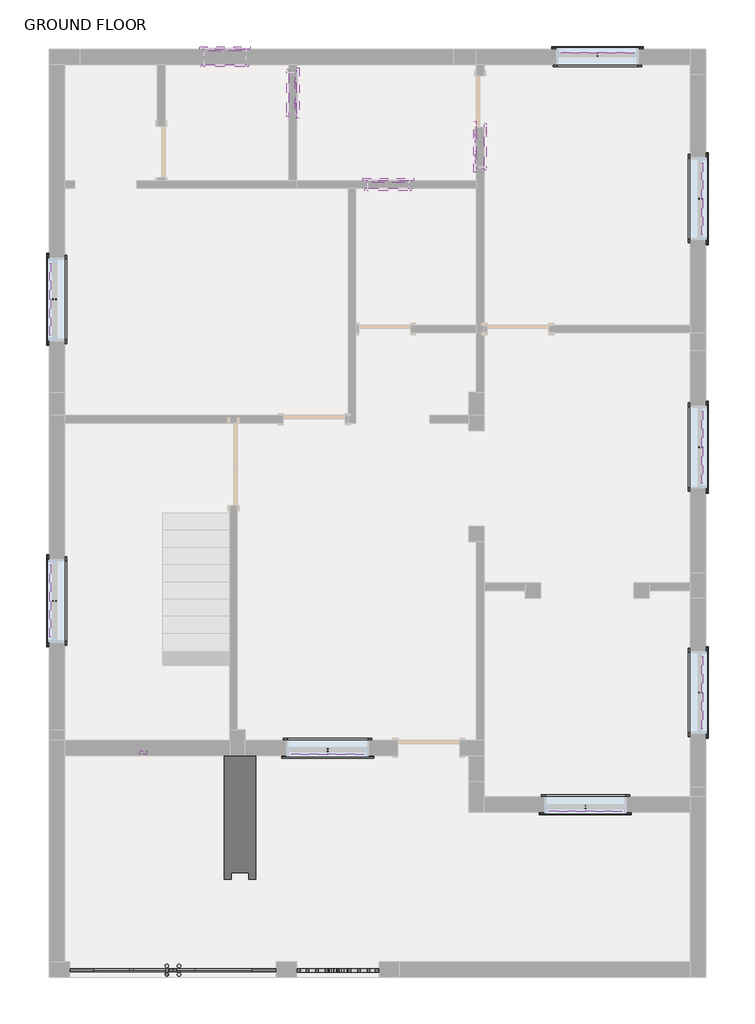
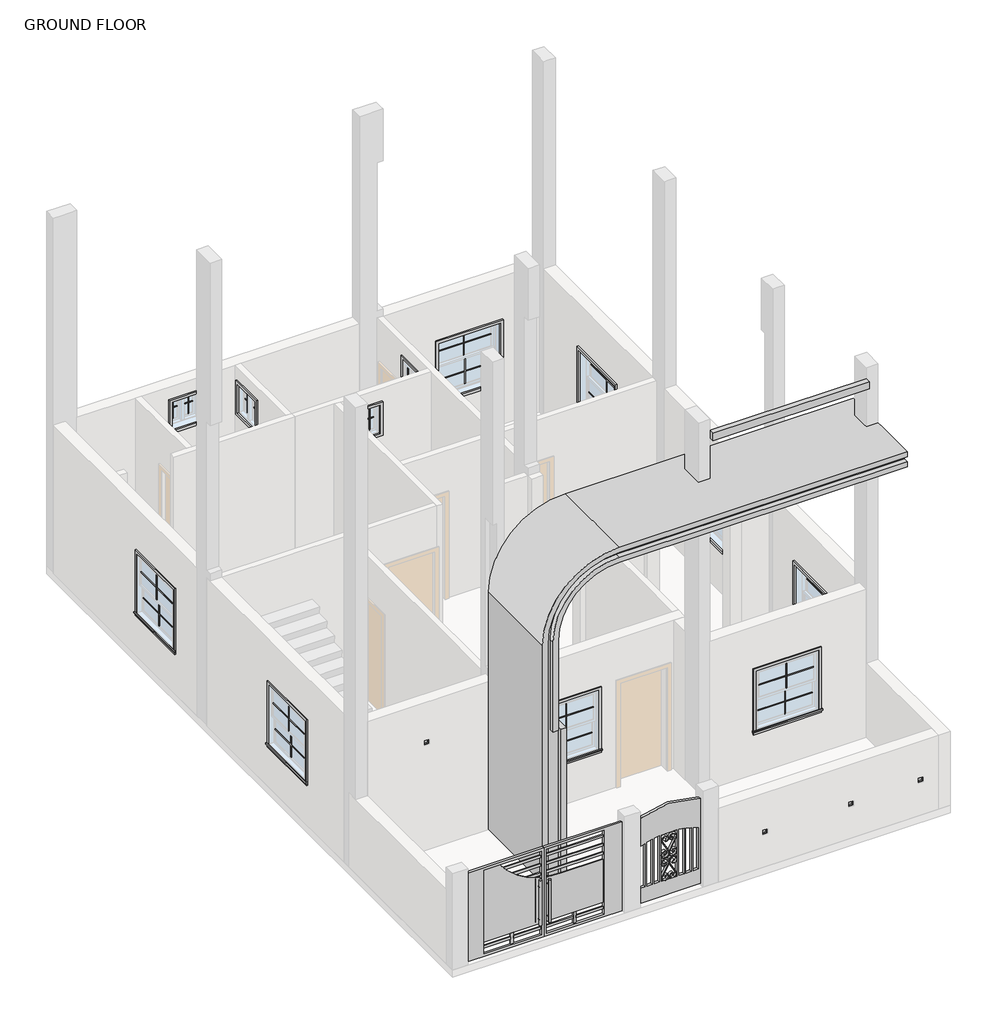
# One storey, part 3 of 3: 51 proxies, 4 light fixtures.
"""IFC4 building model written with IfcOpenShell, lengths in millimetres."""

from ifc_helpers import new_model, si_unit, frame, origin, place, context, project, spatial, polyline, circle_curve, outline, extrude, transform, mapped, element, save
from ifc_brep_helpers import plane_surface, cylinder_surface, revolved_surface, advanced_brep
from components import generic_models_d903a639, muntin_pattern_2x2_muntin_pattern_2x2_1e1a1b39, muntin_pattern_2x2_muntin_pattern_2x2_0961b91c, muntin_pattern_2x2_muntin_pattern_2x2_cae9449b, spanish_gate_w_wrought_iron_detail_3643_spanish_gate_w_2ba93c97, trim_window_exterior_flat_with_sill_7cfdd449, trim_window_exterior_flat_with_sill_858dc10d, trim_window_interior_flat_picture_frame_f1e0b15b, trim_window_interior_flat_picture_frame_3927330c, light_fixture_da35b629

model = new_model("IFC4")

# Units and contexts
model_context = context("Model", 3, world=origin())
ifc_project = project(units=[si_unit("LENGTHUNIT", "METRE", prefix="MILLI")], contexts=[model_context])

# Site, building, storey
site = spatial("IfcSite", under=ifc_project)
building = spatial("IfcBuilding", under=site)
storey = spatial("IfcBuildingStorey", under=building, Name="GROUND FLOOR", Elevation=0.0)

# Proxies
placement = place(None, origin())
generic_models_shape = generic_models_d903a639(model_context)
element("IfcBuildingElementProxy", 1, Name="Generic Models", at=placement, inside=storey, context=model_context, shape_type="MappedRepresentation", body=[
    mapped(generic_models_shape, transform((-11061.7029075, -4701.2829343, 0.0), x_axis=(1.0, 0.0, 0.0), y_axis=(0.0, 1.0, 0.0), z_axis=(0.0, 0.0, 1.0))),
])
element("IfcBuildingElementProxy", 2, Name="Generic Models 1 : Generic Models 1", ObjectType="Generic Models 1 : Generic Models 1", at=placement, inside=storey, context=model_context, shape_type="SolidModel", body=[
    extrude(outline(polyline([(-3417.2209734, -2491.4829343), (-6465.2209734, -2491.4829343), (-6465.2209734, -2389.8829343), (-3417.2209734, -2389.8829343), (-3417.2209734, -2491.4829343)])), frame((0.0, 0.0, 7239.8477718), z_axis=(0.0, 0.0, 1.0), x_axis=(1.0, 0.0, 0.0)), (0.0, 0.0, 1.0), 152.4),
    advanced_brep(
    [(-9837.0709734, -3380.4829343, 0.0), (-9837.0709734, -3380.4829343, 3048.0), (-9938.6709734, -3380.4829343, 3048.0), (-9938.6709734, -3380.4829343, 0.0), (-9837.0709734, -1551.6829343, 0.0), (-10300.6209734, -1551.6829343, 0.0), (-10300.6209734, -1551.6829343, 4902.2), (-8802.0209734, -1551.6829343, 6400.8), (-3188.6209734, -1551.6829343, 6400.8), (-3188.6209734, -1551.6829343, 6096.0), (-8802.0209734, -1551.6829343, 6096.0), (-9995.8209734, -1551.6829343, 4902.2), (-9995.8209734, -1551.6829343, 3048.0), (-9837.0709734, -1551.6829343, 3048.0), (-8802.0209734, -3380.4829343, 6096.0), (-9995.8209734, -3380.4829343, 4902.2), (-3188.6209734, -3380.4829343, 6096.0), (-3188.6209734, -3380.4829343, 6400.8), (-3188.6209734, -3380.4829343, 6299.2), (-3188.6209734, -3278.8829343, 6299.2), (-3188.6209734, -3278.8829343, 6197.6), (-3188.6209734, -3380.4829343, 6197.6), (-8802.0209734, -3380.4829343, 6400.8), (-10300.6209734, -3380.4829343, 4902.2), (-10300.6209734, -3380.4829343, 0.0), (-9938.6709734, -3278.8829343, 0.0), (-10199.0209734, -3278.8829343, 0.0), (-10199.0209734, -3380.4829343, 0.0), (-9995.8209734, -3278.8829343, 3048.0), (-9938.6709734, -3278.8829343, 3048.0), (-9995.8209734, -3380.4829343, 3048.0), (-8802.0209734, -3278.8829343, 6299.2), (-10199.0209734, -3278.8829343, 4902.2), (-10097.4209734, -3278.8829343, 3048.0), (-10097.4209734, -3278.8829343, 4902.2), (-8802.0209734, -3278.8829343, 6197.6), (-8802.0209734, -3380.4829343, 6197.6), (-10097.4209734, -3380.4829343, 4902.2), (-10097.4209734, -3380.4829343, 3048.0), (-10199.0209734, -3380.4829343, 4902.2), (-8802.0209734, -3380.4829343, 6299.2)],
    [
        (0, 1),
        (1, 2),
        (2, 3),
        (3, 0),
        (4, 5),
        (5, 6),
        (6, 7, circle_curve(frame((-8802.0209734, -1551.6829343, 4902.2), z_axis=(0.0, 1.0, 0.0), x_axis=(1.0, 0.0, 0.0)), 1498.6)),
        (7, 8),
        (8, 9),
        (9, 10),
        (10, 11, circle_curve(frame((-8802.0209734, -1551.6829343, 4902.2), z_axis=(0.0, -1.0, 0.0), x_axis=(1.0, 0.0, 0.0)), 1193.8)),
        (11, 12),
        (12, 13),
        (13, 4),
        (0, 4),
        (13, 1),
        (14, 15, circle_curve(frame((-8802.0209734, -3380.4829343, 4902.2), z_axis=(0.0, -1.0, 0.0), x_axis=(1.0, 0.0, 0.0)), 1193.8)),
        (15, 11),
        (10, 14),
        (16, 14),
        (9, 16),
        (8, 17),
        (17, 18),
        (18, 19),
        (19, 20),
        (20, 21),
        (21, 16),
        (22, 17),
        (7, 22),
        (23, 22, circle_curve(frame((-8802.0209734, -3380.4829343, 4902.2), z_axis=(0.0, 1.0, 0.0), x_axis=(1.0, 0.0, 0.0)), 1498.6)),
        (6, 23),
        (24, 23),
        (5, 24),
        (3, 25),
        (25, 26),
        (26, 27),
        (27, 24),
        (12, 28),
        (28, 29),
        (29, 2),
        (15, 30),
        (30, 28),
        (19, 31),
        (31, 32, circle_curve(frame((-8802.0209734, -3278.8829343, 4902.2), z_axis=(0.0, -1.0, 0.0), x_axis=(1.0, 0.0, 0.0)), 1397.0)),
        (32, 26),
        (25, 29),
        (28, 33),
        (33, 34),
        (34, 35, circle_curve(frame((-8802.0209734, -3278.8829343, 4902.2), z_axis=(0.0, 1.0, 0.0), x_axis=(1.0, 0.0, 0.0)), 1295.4)),
        (35, 20),
        (36, 21),
        (35, 36),
        (37, 36, circle_curve(frame((-8802.0209734, -3380.4829343, 4902.2), z_axis=(0.0, 1.0, 0.0), x_axis=(1.0, 0.0, 0.0)), 1295.4)),
        (34, 37),
        (38, 37),
        (33, 38),
        (30, 38),
        (39, 27),
        (32, 39),
        (40, 39, circle_curve(frame((-8802.0209734, -3380.4829343, 4902.2), z_axis=(0.0, -1.0, 0.0), x_axis=(1.0, 0.0, 0.0)), 1397.0)),
        (31, 40),
        (18, 40),
    ],
    [
        plane_surface(frame((-9837.0709734, -3380.4829343, 4902.2), z_axis=(0.0, -1.0, 0.0), x_axis=(0.0, 0.0, 1.0))),
        plane_surface(frame((-9837.0709734, -1551.6829343, 4902.2), z_axis=(0.0, 1.0, 0.0), x_axis=(0.0, 0.0, -1.0))),
        plane_surface(frame((-9837.0709734, -3380.4829343, 0.0), z_axis=(1.0, 0.0, 0.0), x_axis=(0.0, 1.0, 0.0))),
        revolved_surface(polyline([(-7608.2209734, -1551.6829343, 4902.2), (-7608.2209734, -3380.4829343, 4902.2)]), (-8802.0209734, -1551.6829343, 4902.2), (0.0, 1.0, 0.0)),
        plane_surface(frame((-8802.0209734, -3380.4829343, 6096.0), z_axis=(0.0, 0.0, -1.0), x_axis=(0.0, 1.0, 0.0))),
        plane_surface(frame((-3188.6209734, -3380.4829343, 6096.0), z_axis=(1.0, 0.0, 0.0), x_axis=(0.0, 1.0, 0.0))),
        plane_surface(frame((-3188.6209734, -3380.4829343, 6400.8), z_axis=(0.0, 0.0, 1.0), x_axis=(0.0, 1.0, 0.0))),
        cylinder_surface(frame((-8802.0209734, -1551.6829343, 4902.2), z_axis=(0.0, -1.0, 0.0), x_axis=(1.0, 0.0, 0.0)), 1498.6),
        plane_surface(frame((-10300.6209734, -3380.4829343, 4902.2), z_axis=(-1.0, 0.0, 0.0), x_axis=(0.0, 1.0, 0.0))),
        plane_surface(frame((-10300.6209734, -3380.4829343, 0.0), z_axis=(0.0, 0.0, -1.0), x_axis=(0.0, 1.0, 0.0))),
        plane_surface(frame((-9837.0709734, -3380.4829343, 3048.0), z_axis=(0.0, 0.0, 1.0), x_axis=(0.0, 1.0, 0.0))),
        plane_surface(frame((-9995.8209734, -3380.4829343, 3048.0), z_axis=(1.0, 0.0, 0.0), x_axis=(0.0, 1.0, 0.0))),
        plane_surface(frame((-3188.6209734, -3278.8829343, 6299.2), z_axis=(0.0, -1.0, 0.0), x_axis=(0.0, 0.0, -1.0))),
        plane_surface(frame((-3188.6209734, -3278.8829343, 6197.6), z_axis=(0.0, 0.0, 1.0), x_axis=(0.0, -1.0, 0.0))),
        cylinder_surface(frame((-8802.0209734, -3380.4829343, 4902.2), z_axis=(0.0, -1.0, 0.0), x_axis=(1.0, 0.0, 0.0)), 1295.4),
        plane_surface(frame((-10097.4209734, -3278.8829343, 4902.2), z_axis=(-1.0, 0.0, 0.0), x_axis=(0.0, -1.0, 0.0))),
        plane_surface(frame((-10097.4209734, -3278.8829343, 3048.0), z_axis=(0.0, 0.0, -1.0), x_axis=(0.0, -1.0, 0.0))),
        plane_surface(frame((-9938.6709734, -3278.8829343, 3048.0), z_axis=(-1.0, 0.0, 0.0), x_axis=(0.0, -1.0, 0.0))),
        plane_surface(frame((-10199.0209734, -3278.8829343, 0.0), z_axis=(1.0, 0.0, 0.0), x_axis=(0.0, -1.0, 0.0))),
        revolved_surface(polyline([(-7405.0209734, -3278.8829343, 4902.2), (-7405.0209734, -3380.4829343, 4902.2)]), (-8802.0209734, -3380.4829343, 4902.2), (0.0, 1.0, 0.0)),
        plane_surface(frame((-8802.0209734, -3278.8829343, 6299.2), z_axis=(0.0, 0.0, -1.0), x_axis=(0.0, -1.0, 0.0))),
    ],
    [
        (0, [[1, 2, 3, 4]]),
        (1, [[5, 6, 7, 8, 9, 10, 11, 12, 13, 14]]),
        (2, [[-1, 15, -14, 16]]),
        (3, [[17, 18, -11, 19]]),
        (4, [[20, -19, -10, 21]]),
        (5, [[-9, 22, 23, 24, 25, 26, 27, -21]]),
        (6, [[28, -22, -8, 29]]),
        (7, [[30, -29, -7, 31]]),
        (8, [[32, -31, -6, 33]]),
        (9, [[-5, -15, -4, 34, 35, 36, 37, -33]]),
        (10, [[-13, 38, 39, 40, -2, -16]]),
        (11, [[41, 42, -38, -12, -18]]),
        (12, [[-25, 43, 44, 45, -35, 46, -39, 47, 48, 49, 50]]),
        (13, [[51, -26, -50, 52]]),
        (14, [[53, -52, -49, 54]]),
        (15, [[55, -54, -48, 56]]),
        (16, [[57, -56, -47, -42]]),
        (17, [[-3, -40, -46, -34]]),
        (18, [[58, -36, -45, 59]]),
        (19, [[60, -59, -44, 61]]),
        (20, [[62, -61, -43, -24]]),
        (0, [[-41, -17, -20, -27, -51, -53, -55, -57]]),
        (0, [[-28, -30, -32, -37, -58, -60, -62, -23]]),
    ],
),
])
muntin_pattern_2x2_muntin_pattern_2x2_shape = muntin_pattern_2x2_muntin_pattern_2x2_1e1a1b39(model_context)
element("IfcBuildingElementProxy", 3, Name="Muntin Pattern_2x2 : Muntin Pattern_2x2", ObjectType="Muntin Pattern_2x2 : Muntin Pattern_2x2", at=placement, inside=storey, context=model_context, shape_type="MappedRepresentation", body=[
    mapped(muntin_pattern_2x2_muntin_pattern_2x2_shape, transform((-8776.6209734, -1516.7579343, 1546.225), x_axis=(-1.0, 0.0, 0.0), y_axis=(0.0, -1.0, 0.0), z_axis=(0.0, 0.0, 1.0))),
])
element("IfcBuildingElementProxy", 4, Name="Muntin Pattern_2x2 : Muntin Pattern_2x2", ObjectType="Muntin Pattern_2x2 : Muntin Pattern_2x2", at=placement, inside=storey, context=model_context, shape_type="MappedRepresentation", body=[
    mapped(muntin_pattern_2x2_muntin_pattern_2x2_shape, transform((-8776.6209734, -1472.3079343, 990.6), x_axis=(-1.0, 0.0, 0.0), y_axis=(0.0, -1.0, 0.0), z_axis=(0.0, 0.0, 1.0))),
])
element("IfcBuildingElementProxy", 5, Name="Muntin Pattern_2x2 : Muntin Pattern_2x2", ObjectType="Muntin Pattern_2x2 : Muntin Pattern_2x2", at=placement, inside=storey, context=model_context, shape_type="MappedRepresentation", body=[
    mapped(muntin_pattern_2x2_muntin_pattern_2x2_shape, transform((-12856.4959734, 734.3170657, 1546.225), x_axis=(0.0, 1.0, 0.0), y_axis=(-1.0, 0.0, 0.0), z_axis=(0.0, 0.0, 1.0))),
])
element("IfcBuildingElementProxy", 6, Name="Muntin Pattern_2x2 : Muntin Pattern_2x2", ObjectType="Muntin Pattern_2x2 : Muntin Pattern_2x2", at=placement, inside=storey, context=model_context, shape_type="MappedRepresentation", body=[
    mapped(muntin_pattern_2x2_muntin_pattern_2x2_shape, transform((-12812.0459734, 734.3170657, 990.6), x_axis=(0.0, 1.0, 0.0), y_axis=(-1.0, 0.0, 0.0), z_axis=(0.0, 0.0, 1.0))),
])
element("IfcBuildingElementProxy", 7, Name="Muntin Pattern_2x2 : Muntin Pattern_2x2", ObjectType="Muntin Pattern_2x2 : Muntin Pattern_2x2", at=placement, inside=storey, context=model_context, shape_type="MappedRepresentation", body=[
    mapped(muntin_pattern_2x2_muntin_pattern_2x2_shape, transform((-12856.4959734, 5192.0170657, 1546.225), x_axis=(0.0, 1.0, 0.0), y_axis=(-1.0, 0.0, 0.0), z_axis=(0.0, 0.0, 1.0))),
])
element("IfcBuildingElementProxy", 8, Name="Muntin Pattern_2x2 : Muntin Pattern_2x2", ObjectType="Muntin Pattern_2x2 : Muntin Pattern_2x2", at=placement, inside=storey, context=model_context, shape_type="MappedRepresentation", body=[
    mapped(muntin_pattern_2x2_muntin_pattern_2x2_shape, transform((-12812.0459734, 5192.0170657, 990.6), x_axis=(0.0, 1.0, 0.0), y_axis=(-1.0, 0.0, 0.0), z_axis=(0.0, 0.0, 1.0))),
])
element("IfcBuildingElementProxy", 9, Name="Muntin Pattern_2x2 : Muntin Pattern_2x2", ObjectType="Muntin Pattern_2x2 : Muntin Pattern_2x2", at=placement, inside=storey, context=model_context, shape_type="MappedRepresentation", body=[
    mapped(muntin_pattern_2x2_muntin_pattern_2x2_shape, transform((-4788.8209734, 8852.7920657, 1546.225), x_axis=(1.0, 0.0, 0.0), y_axis=(0.0, 1.0, 0.0), z_axis=(0.0, 0.0, 1.0))),
])
element("IfcBuildingElementProxy", 10, Name="Muntin Pattern_2x2 : Muntin Pattern_2x2", ObjectType="Muntin Pattern_2x2 : Muntin Pattern_2x2", at=placement, inside=storey, context=model_context, shape_type="MappedRepresentation", body=[
    mapped(muntin_pattern_2x2_muntin_pattern_2x2_shape, transform((-4788.8209734, 8808.3420657, 990.6), x_axis=(1.0, 0.0, 0.0), y_axis=(0.0, 1.0, 0.0), z_axis=(0.0, 0.0, 1.0))),
])
element("IfcBuildingElementProxy", 11, Name="Muntin Pattern_2x2 : Muntin Pattern_2x2", ObjectType="Muntin Pattern_2x2 : Muntin Pattern_2x2", at=placement, inside=storey, context=model_context, shape_type="MappedRepresentation", body=[
    mapped(muntin_pattern_2x2_muntin_pattern_2x2_shape, transform((-3223.5459734, 6677.9170657, 1546.225), x_axis=(0.0, -1.0, 0.0), y_axis=(1.0, 0.0, 0.0), z_axis=(0.0, 0.0, 1.0))),
])
element("IfcBuildingElementProxy", 12, Name="Muntin Pattern_2x2 : Muntin Pattern_2x2", ObjectType="Muntin Pattern_2x2 : Muntin Pattern_2x2", at=placement, inside=storey, context=model_context, shape_type="MappedRepresentation", body=[
    mapped(muntin_pattern_2x2_muntin_pattern_2x2_shape, transform((-3267.9959734, 6677.9170657, 990.6), x_axis=(0.0, -1.0, 0.0), y_axis=(1.0, 0.0, 0.0), z_axis=(0.0, 0.0, 1.0))),
])
element("IfcBuildingElementProxy", 13, Name="Muntin Pattern_2x2 : Muntin Pattern_2x2", ObjectType="Muntin Pattern_2x2 : Muntin Pattern_2x2", at=placement, inside=storey, context=model_context, shape_type="MappedRepresentation", body=[
    mapped(muntin_pattern_2x2_muntin_pattern_2x2_shape, transform((-3223.5459734, 3007.6170657, 1546.225), x_axis=(0.0, -1.0, 0.0), y_axis=(1.0, 0.0, 0.0), z_axis=(0.0, 0.0, 1.0))),
])
element("IfcBuildingElementProxy", 14, Name="Muntin Pattern_2x2 : Muntin Pattern_2x2", ObjectType="Muntin Pattern_2x2 : Muntin Pattern_2x2", at=placement, inside=storey, context=model_context, shape_type="MappedRepresentation", body=[
    mapped(muntin_pattern_2x2_muntin_pattern_2x2_shape, transform((-3267.9959734, 3007.6170657, 990.6), x_axis=(0.0, -1.0, 0.0), y_axis=(1.0, 0.0, 0.0), z_axis=(0.0, 0.0, 1.0))),
])
element("IfcBuildingElementProxy", 15, Name="Muntin Pattern_2x2 : Muntin Pattern_2x2", ObjectType="Muntin Pattern_2x2 : Muntin Pattern_2x2", at=placement, inside=storey, context=model_context, shape_type="MappedRepresentation", body=[
    mapped(muntin_pattern_2x2_muntin_pattern_2x2_shape, transform((-3223.5459734, -618.2329343, 1546.225), x_axis=(0.0, -1.0, 0.0), y_axis=(1.0, 0.0, 0.0), z_axis=(0.0, 0.0, 1.0))),
])
element("IfcBuildingElementProxy", 16, Name="Muntin Pattern_2x2 : Muntin Pattern_2x2", ObjectType="Muntin Pattern_2x2 : Muntin Pattern_2x2", at=placement, inside=storey, context=model_context, shape_type="MappedRepresentation", body=[
    mapped(muntin_pattern_2x2_muntin_pattern_2x2_shape, transform((-3267.9959734, -618.2329343, 990.6), x_axis=(0.0, -1.0, 0.0), y_axis=(1.0, 0.0, 0.0), z_axis=(0.0, 0.0, 1.0))),
])
element("IfcBuildingElementProxy", 17, Name="Muntin Pattern_2x2 : Muntin Pattern_2x2", ObjectType="Muntin Pattern_2x2 : Muntin Pattern_2x2", at=placement, inside=storey, context=model_context, shape_type="MappedRepresentation", body=[
    mapped(muntin_pattern_2x2_muntin_pattern_2x2_shape, transform((-4966.6209734, -2354.9579343, 1546.225), x_axis=(-1.0, 0.0, 0.0), y_axis=(0.0, -1.0, 0.0), z_axis=(0.0, 0.0, 1.0))),
])
element("IfcBuildingElementProxy", 18, Name="Muntin Pattern_2x2 : Muntin Pattern_2x2", ObjectType="Muntin Pattern_2x2 : Muntin Pattern_2x2", at=placement, inside=storey, context=model_context, shape_type="MappedRepresentation", body=[
    mapped(muntin_pattern_2x2_muntin_pattern_2x2_shape, transform((-4966.6209734, -2310.5079343, 990.6), x_axis=(-1.0, 0.0, 0.0), y_axis=(0.0, -1.0, 0.0), z_axis=(0.0, 0.0, 1.0))),
])
muntin_pattern_2x2_muntin_pattern_2x2_2_shape = muntin_pattern_2x2_muntin_pattern_2x2_0961b91c(model_context)
element("IfcBuildingElementProxy", 19, Name="Muntin Pattern_2x2 : Muntin Pattern_2x2", ObjectType="Muntin Pattern_2x2 : Muntin Pattern_2x2", at=placement, inside=storey, context=model_context, shape_type="MappedRepresentation", body=[
    mapped(muntin_pattern_2x2_muntin_pattern_2x2_2_shape, transform((-8032.0834734, 6935.0920657, 2203.45), x_axis=(1.0, 0.0, 0.0), y_axis=(0.0, 1.0, 0.0), z_axis=(0.0, 0.0, 1.0))),
])
element("IfcBuildingElementProxy", 20, Name="Muntin Pattern_2x2 : Muntin Pattern_2x2", ObjectType="Muntin Pattern_2x2 : Muntin Pattern_2x2", at=placement, inside=storey, context=model_context, shape_type="MappedRepresentation", body=[
    mapped(muntin_pattern_2x2_muntin_pattern_2x2_2_shape, transform((-9243.3459734, 8390.8295657, 2203.45), x_axis=(0.0, -1.0, 0.0), y_axis=(1.0, 0.0, 0.0), z_axis=(0.0, 0.0, 1.0))),
])
element("IfcBuildingElementProxy", 21, Name="Muntin Pattern_2x2 : Muntin Pattern_2x2", ObjectType="Muntin Pattern_2x2 : Muntin Pattern_2x2", at=placement, inside=storey, context=model_context, shape_type="MappedRepresentation", body=[
    mapped(muntin_pattern_2x2_muntin_pattern_2x2_2_shape, transform((-10445.0834734, 8878.1920657, 2203.45), x_axis=(1.0, 0.0, 0.0), y_axis=(0.0, 1.0, 0.0), z_axis=(0.0, 0.0, 1.0))),
])
element("IfcBuildingElementProxy", 22, Name="Muntin Pattern_2x2 : Muntin Pattern_2x2", ObjectType="Muntin Pattern_2x2 : Muntin Pattern_2x2", at=placement, inside=storey, context=model_context, shape_type="MappedRepresentation", body=[
    mapped(muntin_pattern_2x2_muntin_pattern_2x2_2_shape, transform((-6569.9959734, 7295.4545657, 2203.45), x_axis=(0.0, 1.0, 0.0), y_axis=(-1.0, 0.0, 0.0), z_axis=(0.0, 0.0, 1.0))),
])
muntin_pattern_2x2_muntin_pattern_2x2_3_shape = muntin_pattern_2x2_muntin_pattern_2x2_cae9449b(model_context)
element("IfcBuildingElementProxy", 23, Name="Muntin Pattern_2x2 : Muntin Pattern_2x2", ObjectType="Muntin Pattern_2x2 : Muntin Pattern_2x2", at=placement, inside=storey, context=model_context, shape_type="MappedRepresentation", body=[
    mapped(muntin_pattern_2x2_muntin_pattern_2x2_3_shape, transform((-7730.4584734, 6935.0920657, 2203.45), x_axis=(-1.0, 0.0, 0.0), y_axis=(0.0, -1.0, 0.0), z_axis=(0.0, 0.0, 1.0))),
])
element("IfcBuildingElementProxy", 24, Name="Muntin Pattern_2x2 : Muntin Pattern_2x2", ObjectType="Muntin Pattern_2x2 : Muntin Pattern_2x2", at=placement, inside=storey, context=model_context, shape_type="MappedRepresentation", body=[
    mapped(muntin_pattern_2x2_muntin_pattern_2x2_3_shape, transform((-9243.3459734, 8089.2045657, 2203.45), x_axis=(0.0, 1.0, 0.0), y_axis=(-1.0, 0.0, 0.0), z_axis=(0.0, 0.0, 1.0))),
])
element("IfcBuildingElementProxy", 25, Name="Muntin Pattern_2x2 : Muntin Pattern_2x2", ObjectType="Muntin Pattern_2x2 : Muntin Pattern_2x2", at=placement, inside=storey, context=model_context, shape_type="MappedRepresentation", body=[
    mapped(muntin_pattern_2x2_muntin_pattern_2x2_3_shape, transform((-10143.4584734, 8878.1920657, 2203.45), x_axis=(-1.0, 0.0, 0.0), y_axis=(0.0, -1.0, 0.0), z_axis=(0.0, 0.0, 1.0))),
])
element("IfcBuildingElementProxy", 26, Name="Muntin Pattern_2x2 : Muntin Pattern_2x2", ObjectType="Muntin Pattern_2x2 : Muntin Pattern_2x2", at=placement, inside=storey, context=model_context, shape_type="MappedRepresentation", body=[
    mapped(muntin_pattern_2x2_muntin_pattern_2x2_3_shape, transform((-6569.9959734, 7597.0795657, 2203.45), x_axis=(0.0, -1.0, 0.0), y_axis=(1.0, 0.0, 0.0), z_axis=(0.0, 0.0, 1.0))),
])
spanish_gate_w_wrought_iron_detail_3643_spanish_gate_w_shape = spanish_gate_w_wrought_iron_detail_3643_spanish_gate_w_2ba93c97(model_context)
element("IfcBuildingElementProxy", 27, Name="Spanish_Gate_w_wrought_iron_detail_3643 : Spanish_Gate_w_wrought_iron_detail_3643", ObjectType="Spanish_Gate_w_wrought_iron_detail_3643 : Spanish_Gate_w_wrought_iron_detail_3643", at=placement, inside=storey, context=model_context, shape_type="MappedRepresentation", body=[
    mapped(spanish_gate_w_wrought_iron_detail_3643_spanish_gate_w_shape, transform((-8624.2209734, -4701.2829343, 304.8), x_axis=(1.0, 0.0, 0.0), y_axis=(0.0, 1.0, 0.0), z_axis=(0.0, 0.0, 1.0))),
])
trim_window_exterior_flat_with_sill_shape = trim_window_exterior_flat_with_sill_7cfdd449(model_context)
element("IfcBuildingElementProxy", 28, Name="Trim-Window-Exterior-Flat : with Sill", ObjectType="Trim-Window-Exterior-Flat : with Sill", at=placement, inside=storey, context=model_context, shape_type="MappedRepresentation", body=[
    mapped(trim_window_exterior_flat_with_sill_shape, transform((-8776.6209734, -1551.6829343, 2133.6), x_axis=(1.0, 0.0, 0.0), y_axis=(0.0, 0.0, 1.0), z_axis=(0.0, -1.0, 0.0))),
])
element("IfcBuildingElementProxy", 29, Name="Trim-Window-Exterior-Flat : with Sill", ObjectType="Trim-Window-Exterior-Flat : with Sill", at=placement, inside=storey, context=model_context, shape_type="MappedRepresentation", body=[
    mapped(trim_window_exterior_flat_with_sill_shape, transform((-12891.4209734, 734.3170657, 2133.6), x_axis=(0.0, -1.0, 0.0), y_axis=(0.0, 0.0, 1.0), z_axis=(-1.0, 0.0, 0.0))),
])
element("IfcBuildingElementProxy", 30, Name="Trim-Window-Exterior-Flat : with Sill", ObjectType="Trim-Window-Exterior-Flat : with Sill", at=placement, inside=storey, context=model_context, shape_type="MappedRepresentation", body=[
    mapped(trim_window_exterior_flat_with_sill_shape, transform((-12891.4209734, 5192.0170657, 2133.6), x_axis=(0.0, -1.0, 0.0), y_axis=(0.0, 0.0, 1.0), z_axis=(-1.0, 0.0, 0.0))),
])
element("IfcBuildingElementProxy", 31, Name="Trim-Window-Exterior-Flat : with Sill", ObjectType="Trim-Window-Exterior-Flat : with Sill", at=placement, inside=storey, context=model_context, shape_type="MappedRepresentation", body=[
    mapped(trim_window_exterior_flat_with_sill_shape, transform((-4788.8209734, 8887.7170657, 2133.6), x_axis=(-1.0, 0.0, 0.0), y_axis=(0.0, 0.0, 1.0), z_axis=(0.0, 1.0, 0.0))),
])
element("IfcBuildingElementProxy", 32, Name="Trim-Window-Exterior-Flat : with Sill", ObjectType="Trim-Window-Exterior-Flat : with Sill", at=placement, inside=storey, context=model_context, shape_type="MappedRepresentation", body=[
    mapped(trim_window_exterior_flat_with_sill_shape, transform((-3188.6209734, 6677.9170657, 2133.6), x_axis=(0.0, 1.0, 0.0), y_axis=(0.0, 0.0, 1.0), z_axis=(1.0, 0.0, 0.0))),
])
element("IfcBuildingElementProxy", 33, Name="Trim-Window-Exterior-Flat : with Sill", ObjectType="Trim-Window-Exterior-Flat : with Sill", at=placement, inside=storey, context=model_context, shape_type="MappedRepresentation", body=[
    mapped(trim_window_exterior_flat_with_sill_shape, transform((-3188.6209734, 3007.6170657, 2133.6), x_axis=(0.0, 1.0, 0.0), y_axis=(0.0, 0.0, 1.0), z_axis=(1.0, 0.0, 0.0))),
])
element("IfcBuildingElementProxy", 34, Name="Trim-Window-Exterior-Flat : with Sill", ObjectType="Trim-Window-Exterior-Flat : with Sill", at=placement, inside=storey, context=model_context, shape_type="MappedRepresentation", body=[
    mapped(trim_window_exterior_flat_with_sill_shape, transform((-3188.6209734, -618.2329343, 2133.6), x_axis=(0.0, 1.0, 0.0), y_axis=(0.0, 0.0, 1.0), z_axis=(1.0, 0.0, 0.0))),
])
element("IfcBuildingElementProxy", 35, Name="Trim-Window-Exterior-Flat : with Sill", ObjectType="Trim-Window-Exterior-Flat : with Sill", at=placement, inside=storey, context=model_context, shape_type="MappedRepresentation", body=[
    mapped(trim_window_exterior_flat_with_sill_shape, transform((-4966.6209734, -2389.8829343, 2133.6), x_axis=(1.0, 0.0, 0.0), y_axis=(0.0, 0.0, 1.0), z_axis=(0.0, -1.0, 0.0))),
])
trim_window_exterior_flat_with_sill_2_shape = trim_window_exterior_flat_with_sill_858dc10d(model_context)
element("IfcBuildingElementProxy", 36, Name="Trim-Window-Exterior-Flat : with Sill", ObjectType="Trim-Window-Exterior-Flat : with Sill", at=placement, inside=storey, context=model_context, shape_type="MappedRepresentation", body=[
    mapped(trim_window_exterior_flat_with_sill_2_shape, transform((-7881.2709734, 6944.6170657, 2743.2), x_axis=(-1.0, 0.0, 0.0), y_axis=(0.0, 0.0, 1.0), z_axis=(0.0, 1.0, 0.0))),
])
element("IfcBuildingElementProxy", 37, Name="Trim-Window-Exterior-Flat : with Sill", ObjectType="Trim-Window-Exterior-Flat : with Sill", at=placement, inside=storey, context=model_context, shape_type="MappedRepresentation", body=[
    mapped(trim_window_exterior_flat_with_sill_2_shape, transform((-9233.8209734, 8240.0170657, 2743.2), x_axis=(0.0, 1.0, 0.0), y_axis=(0.0, 0.0, 1.0), z_axis=(1.0, 0.0, 0.0))),
])
element("IfcBuildingElementProxy", 38, Name="Trim-Window-Exterior-Flat : with Sill", ObjectType="Trim-Window-Exterior-Flat : with Sill", at=placement, inside=storey, context=model_context, shape_type="MappedRepresentation", body=[
    mapped(trim_window_exterior_flat_with_sill_2_shape, transform((-10294.2709734, 8887.7170657, 2743.2), x_axis=(-1.0, 0.0, 0.0), y_axis=(0.0, 0.0, 1.0), z_axis=(0.0, 1.0, 0.0))),
])
element("IfcBuildingElementProxy", 39, Name="Trim-Window-Exterior-Flat : with Sill", ObjectType="Trim-Window-Exterior-Flat : with Sill", at=placement, inside=storey, context=model_context, shape_type="MappedRepresentation", body=[
    mapped(trim_window_exterior_flat_with_sill_2_shape, transform((-6579.5209734, 7446.2670657, 2743.2), x_axis=(0.0, -1.0, 0.0), y_axis=(0.0, 0.0, 1.0), z_axis=(-1.0, 0.0, 0.0))),
])
trim_window_interior_flat_picture_frame_shape = trim_window_interior_flat_picture_frame_f1e0b15b(model_context)
element("IfcBuildingElementProxy", 40, Name="Trim-Window-Interior-Flat : Picture Frame", ObjectType="Trim-Window-Interior-Flat : Picture Frame", at=placement, inside=storey, context=model_context, shape_type="MappedRepresentation", body=[
    mapped(trim_window_interior_flat_picture_frame_shape, transform((-8776.6209734, -1323.0829343, 2133.6), x_axis=(-1.0, 0.0, 0.0), y_axis=(0.0, 0.0, 1.0), z_axis=(0.0, 1.0, 0.0))),
])
element("IfcBuildingElementProxy", 41, Name="Trim-Window-Interior-Flat : Picture Frame", ObjectType="Trim-Window-Interior-Flat : Picture Frame", at=placement, inside=storey, context=model_context, shape_type="MappedRepresentation", body=[
    mapped(trim_window_interior_flat_picture_frame_shape, transform((-12662.8209734, 734.3170657, 2133.6), x_axis=(0.0, 1.0, 0.0), y_axis=(0.0, 0.0, 1.0), z_axis=(1.0, 0.0, 0.0))),
])
element("IfcBuildingElementProxy", 42, Name="Trim-Window-Interior-Flat : Picture Frame", ObjectType="Trim-Window-Interior-Flat : Picture Frame", at=placement, inside=storey, context=model_context, shape_type="MappedRepresentation", body=[
    mapped(trim_window_interior_flat_picture_frame_shape, transform((-12662.8209734, 5192.0170657, 2133.6), x_axis=(0.0, 1.0, 0.0), y_axis=(0.0, 0.0, 1.0), z_axis=(1.0, 0.0, 0.0))),
])
element("IfcBuildingElementProxy", 43, Name="Trim-Window-Interior-Flat : Picture Frame", ObjectType="Trim-Window-Interior-Flat : Picture Frame", at=placement, inside=storey, context=model_context, shape_type="MappedRepresentation", body=[
    mapped(trim_window_interior_flat_picture_frame_shape, transform((-4788.8209734, 8659.1170657, 2133.6), x_axis=(1.0, 0.0, 0.0), y_axis=(0.0, 0.0, 1.0), z_axis=(0.0, -1.0, 0.0))),
])
element("IfcBuildingElementProxy", 44, Name="Trim-Window-Interior-Flat : Picture Frame", ObjectType="Trim-Window-Interior-Flat : Picture Frame", at=placement, inside=storey, context=model_context, shape_type="MappedRepresentation", body=[
    mapped(trim_window_interior_flat_picture_frame_shape, transform((-3417.2209734, 6677.9170657, 2133.6), x_axis=(0.0, -1.0, 0.0), y_axis=(0.0, 0.0, 1.0), z_axis=(-1.0, 0.0, 0.0))),
])
element("IfcBuildingElementProxy", 45, Name="Trim-Window-Interior-Flat : Picture Frame", ObjectType="Trim-Window-Interior-Flat : Picture Frame", at=placement, inside=storey, context=model_context, shape_type="MappedRepresentation", body=[
    mapped(trim_window_interior_flat_picture_frame_shape, transform((-3417.2209734, 3007.6170657, 2133.6), x_axis=(0.0, -1.0, 0.0), y_axis=(0.0, 0.0, 1.0), z_axis=(-1.0, 0.0, 0.0))),
])
element("IfcBuildingElementProxy", 46, Name="Trim-Window-Interior-Flat : Picture Frame", ObjectType="Trim-Window-Interior-Flat : Picture Frame", at=placement, inside=storey, context=model_context, shape_type="MappedRepresentation", body=[
    mapped(trim_window_interior_flat_picture_frame_shape, transform((-3417.2209734, -618.2329343, 2133.6), x_axis=(0.0, -1.0, 0.0), y_axis=(0.0, 0.0, 1.0), z_axis=(-1.0, 0.0, 0.0))),
])
element("IfcBuildingElementProxy", 47, Name="Trim-Window-Interior-Flat : Picture Frame", ObjectType="Trim-Window-Interior-Flat : Picture Frame", at=placement, inside=storey, context=model_context, shape_type="MappedRepresentation", body=[
    mapped(trim_window_interior_flat_picture_frame_shape, transform((-4966.6209734, -2161.2829343, 2133.6), x_axis=(-1.0, 0.0, 0.0), y_axis=(0.0, 0.0, 1.0), z_axis=(0.0, 1.0, 0.0))),
])
trim_window_interior_flat_picture_frame_2_shape = trim_window_interior_flat_picture_frame_3927330c(model_context)
element("IfcBuildingElementProxy", 48, Name="Trim-Window-Interior-Flat : Picture Frame", ObjectType="Trim-Window-Interior-Flat : Picture Frame", at=placement, inside=storey, context=model_context, shape_type="MappedRepresentation", body=[
    mapped(trim_window_interior_flat_picture_frame_2_shape, transform((-7881.2709734, 6830.3170657, 2743.2), x_axis=(1.0, 0.0, 0.0), y_axis=(0.0, 0.0, 1.0), z_axis=(0.0, -1.0, 0.0))),
])
element("IfcBuildingElementProxy", 49, Name="Trim-Window-Interior-Flat : Picture Frame", ObjectType="Trim-Window-Interior-Flat : Picture Frame", at=placement, inside=storey, context=model_context, shape_type="MappedRepresentation", body=[
    mapped(trim_window_interior_flat_picture_frame_2_shape, transform((-9348.1209734, 8240.0170657, 2743.2), x_axis=(0.0, -1.0, 0.0), y_axis=(0.0, 0.0, 1.0), z_axis=(-1.0, 0.0, 0.0))),
])
element("IfcBuildingElementProxy", 50, Name="Trim-Window-Interior-Flat : Picture Frame", ObjectType="Trim-Window-Interior-Flat : Picture Frame", at=placement, inside=storey, context=model_context, shape_type="MappedRepresentation", body=[
    mapped(trim_window_interior_flat_picture_frame_2_shape, transform((-10294.2709734, 8659.1170657, 2743.2), x_axis=(1.0, 0.0, 0.0), y_axis=(0.0, 0.0, 1.0), z_axis=(0.0, -1.0, 0.0))),
])
element("IfcBuildingElementProxy", 51, Name="Trim-Window-Interior-Flat : Picture Frame", ObjectType="Trim-Window-Interior-Flat : Picture Frame", at=placement, inside=storey, context=model_context, shape_type="MappedRepresentation", body=[
    mapped(trim_window_interior_flat_picture_frame_2_shape, transform((-6465.2209734, 7446.2670657, 2743.2), x_axis=(0.0, 1.0, 0.0), y_axis=(0.0, 0.0, 1.0), z_axis=(1.0, 0.0, 0.0))),
])

# Light fixtures
light_fixture_shape = light_fixture_da35b629(model_context)
element("IfcLightFixture", 52, at=placement, inside=storey, context=model_context, shape_type="MappedRepresentation", body=[
    mapped(light_fixture_shape, transform((-11537.1266361, -1437.3829343, 217.5734947), x_axis=(-1.0, 0.0, 0.0), y_axis=(0.0, -1.0, 0.0), z_axis=(0.0, 0.0, 1.0))),
])
element("IfcLightFixture", 53, at=placement, inside=storey, context=model_context, shape_type="MappedRepresentation", body=[
    mapped(light_fixture_shape, transform((-6831.7766361, -4713.9829343, -1286.005654), x_axis=(-1.0, 0.0, 0.0), y_axis=(0.0, -1.0, 0.0), z_axis=(0.0, 0.0, 1.0))),
])
element("IfcLightFixture", 54, at=placement, inside=storey, context=model_context, shape_type="MappedRepresentation", body=[
    mapped(light_fixture_shape, transform((-5155.3766361, -4713.9829343, -1298.0804736), x_axis=(-1.0, 0.0, 0.0), y_axis=(0.0, -1.0, 0.0), z_axis=(0.0, 0.0, 1.0))),
])
element("IfcLightFixture", 55, at=placement, inside=storey, context=model_context, shape_type="MappedRepresentation", body=[
    mapped(light_fixture_shape, transform((-3796.4766361, -4713.9829343, -1280.3135665), x_axis=(-1.0, 0.0, 0.0), y_axis=(0.0, -1.0, 0.0), z_axis=(0.0, 0.0, 1.0))),
])

save(model, "model.ifc")

# Revit data of these elements
# Type
#   sheet = none
#   pipe = none
#   handal = none
#   faram = none
#   Default Elevation = 0
# Type "Muntin Pattern_2x2 : Muntin Pattern_2x2"
#   Width [instance default] = 4' - 0"
#   Thickness = 0' - 0 1/2"
#   Height [instance default] = 4' - 0"
#   Distance = 0' - 0 3/4"
#   Interior Material [instance default] = none
#   Exterior Material [instance default] = none
#   Default Elevation = 0
# Type "Spanish_Gate_w_wrought_iron_detail_3643 : Spanish_Gate_w_wrought_iron_detail_3643"
#   Default Elevation = 0
# Type "Trim-Window-Exterior-Flat : with Sill"
#   Trim Width = 0' - 2 1/4"
#   Trim Thickness_Picture Frame = 0' - 1 1/4"
#   Trim Thickness_with Sill = 0' - 0 3/4"
#   Sill Thickness = 0' - 1 1/4"
#   Opening Width [instance default] = 2' - 0"
#   Opening Height [instance default] = 3' - 0"
#   Default Elevation = 4' - 0"
#   Sill = yes
#   Picture Frame = no
#   Trim Material [instance default] = none
# Type "Trim-Window-Interior-Flat : Picture Frame"
#   Trim Thickness_Picture Frame = 0' - 1 1/4"
#   Trim Width = 0' - 2 1/4"
#   Trim Thickness_with Sill = 0' - 0 3/4"
#   Sill Thickness = 0' - 1 1/4"
#   Opening Width [instance default] = 2' - 0"
#   Opening Height [instance default] = 3' - 0"
#   Default Elevation = 4' - 0"
#   Sill = no
#   Picture Frame = yes
#   Trim Material [instance default] = none
# Type
#   rahmen dicke = 0' - 0.98819"
#   rahmen breite(okvir) = 0' - 0.55118"
#   rahmen breite = 0' - 1.9685"
#   glas dicke = 0' - 0.82349"
#   abstand von wand (lichtquelle) = 0' - 2.76378"
#   Wattage = 20.16 W
#   Emit from Circle Diameter = 0' - 4.31496"
#   built-in parameter 1150110 = 1 (stored number, unit not read)
#   built-in parameter 1114217 = 1 (stored number, unit not read)
#   built-in parameter 1150109 = 1 (stored number, unit not read)
#   built-in parameter 1150113 = 1 (stored number, unit not read)
#   Lumens = 2994.61 lm
#   built-in parameter 1150115 = 1 (stored number, unit not read)
#   built-in parameter 1150105 = 953.213 (stored number, unit not read)
#   Light Source Symbol Size = 2' - 0"
#   built-in parameter 1150112 = 1 (stored number, unit not read)
#   built-in parameter 1150114 = 1 (stored number, unit not read)
#   built-in parameter 1150107 = 3000 (stored number, unit not read)
#   built-in parameter 1150106 = 9.53213 (stored number, unit not read)
#   built-in parameter 1150104 = 13.8 (stored number, unit not read)
#   built-in parameter 1114218 = 1 (stored number, unit not read)
#   built-in parameter 1150133 = 10 (stored number, unit not read)
#   Emit Shape Visible in Rendering = yes
#   Color Filter = 16744448
#   rahmen material = rahmen material
#   glass material = glas material
#   Dimming Lamp Color Temperature Shift = (empty or 0)
#   Default Elevation = 0
# Element 1 (IfcBuildingElementProxy)
#   Phase Created = New Construction
# Element 2 (IfcBuildingElementProxy, "Generic Models 1 : Generic Models 1")
#   Phase Created = New Construction
#   Materials on its faces: "Earth", "Wood - Stained"
# Elements 3, 4, 5, 6, 7, 8, 9, 10, 11, 12, 13, 14, 15, 16, 17, 18 (IfcBuildingElementProxy, "Muntin Pattern_2x2 : Muntin Pattern_2x2")
#   Width = 3' - 6"
#   Height = 1' - 8 1/8"
#   Interior Material = Wood - Stained
#   Exterior Material = Clad - White
#   Phase Created = New Construction
#   Materials on its faces: "Clad - White", "Wood - Stained"
# Elements 19, 20, 21, 22, 23, 24, 25, 26 (IfcBuildingElementProxy, "Muntin Pattern_2x2 : Muntin Pattern_2x2")
#   Width = 0' - 6 5/8"
#   Height = 1' - 6 1/2"
#   Interior Material = Wood - Stained
#   Exterior Material = Clad - White
#   Phase Created = New Construction
#   Materials on its faces: "Clad - White", "Wood - Stained"
# Element 27 (IfcBuildingElementProxy, "Spanish_Gate_w_wrought_iron_detail_3643 : Spanish_Gate_w_wrought_iron_detail_3643")
#   Phase Created = New Construction
#   Materials on its faces: "iron"
# Elements 28, 29, 30, 31, 32, 33, 34, 35 (IfcBuildingElementProxy, "Trim-Window-Exterior-Flat : with Sill")
#   Opening Width = 4' - 0"
#   Opening Height = 4' - 0"
#   Trim Material = Clad - White
#   Phase Created = New Construction
#   Materials on its faces: "Clad - White"
# Elements 36, 37, 38, 39 (IfcBuildingElementProxy, "Trim-Window-Exterior-Flat : with Sill")
#   Opening Width = 2' - 0"
#   Opening Height = 2' - 0"
#   Trim Material = Clad - White
#   Phase Created = New Construction
#   Materials on its faces: "Clad - White"
# Elements 40, 41, 42, 43, 44, 45, 46, 47 (IfcBuildingElementProxy, "Trim-Window-Interior-Flat : Picture Frame")
#   Opening Width = 4' - 0"
#   Opening Height = 4' - 0"
#   Trim Material = Wood - Stained
#   Phase Created = New Construction
#   Materials on its faces: "Wood - Stained"
# Elements 48, 49, 50, 51 (IfcBuildingElementProxy, "Trim-Window-Interior-Flat : Picture Frame")
#   Opening Width = 2' - 0"
#   Opening Height = 2' - 0"
#   Trim Material = Wood - Stained
#   Phase Created = New Construction
#   Materials on its faces: "Wood - Stained"
# Element 52 (IfcLightFixture)
#   Mark = "4"
#   Phase Created = New Construction
#   Materials on its faces: "rahmen material", "glas material"
# Element 53 (IfcLightFixture)
#   Mark = "5"
#   Phase Created = New Construction
#   Materials on its faces: "rahmen material", "glas material"
# Element 54 (IfcLightFixture)
#   Mark = "6"
#   Phase Created = New Construction
#   Materials on its faces: "rahmen material", "glas material"
# Element 55 (IfcLightFixture)
#   Mark = "7"
#   Phase Created = New Construction
#   Materials on its faces: "rahmen material", "glas material"
# Materials
#   "rahmen material": class "Glas", colour RGB 0 0 255, transparency 0.75
#   "glas material": class "Glas", colour RGB 0 128 192, transparency 0.9
#   "Earth": class "Generic", colour RGB 97 75 62, transparency 0, Description = "Soil", Cost = 0
#   "Wood - Stained": class "Wood", colour RGB 224 178 126, transparency 0, Cost = 0
#   "Clad - White": class "Wood", colour RGB 242 242 238, transparency 0, Cost = 0
#   "iron": colour RGB 49 49 49, transparency 0
